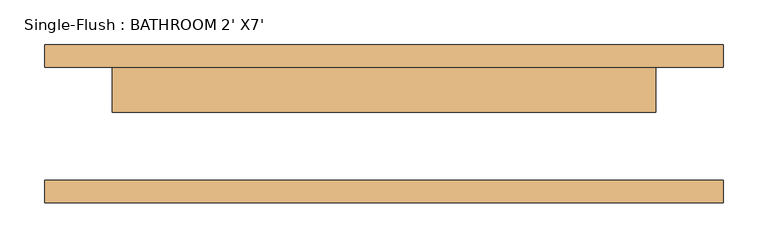
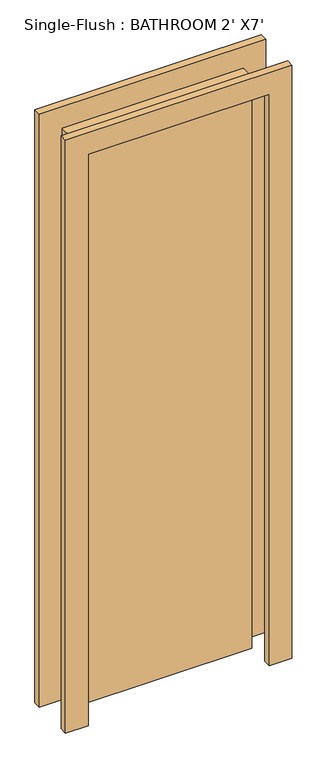
"""IFC4 building model written with IfcOpenShell, lengths in millimetres: door geometry, Single-Flush : BATHROOM 2' X7'."""

from ifc_helpers import new_model, si_unit, frame, origin, origin_with_axes, place, context, project, spatial, polyline, outline, extrude, source, transform, mapped, element, save


def single_flush_bathroom_2_x7_025d1c86(model_context):
    return source(origin(), model_context, "Body", "SweptSolid", [
        extrude(outline(polyline([(2108.2, -381.0), (0.0, -381.0), (0.0, -304.8), (2032.0, -304.8), (2032.0, 304.8), (0.0, 304.8), (0.0, 381.0), (2108.2, 381.0), (2108.2, -381.0)])), frame((0.0, 63.5, 0.0), z_axis=(0.0, 1.0, 0.0), x_axis=(0.0, 0.0, 1.0)), (0.0, 0.0, 1.0), 25.4),
        extrude(outline(polyline([(2108.2, 381.0), (2108.2, -381.0), (0.0, -381.0), (0.0, -304.8), (2032.0, -304.8), (2032.0, 304.8), (0.0, 304.8), (0.0, 381.0), (2108.2, 381.0)])), frame((0.0, -88.9, 0.0), z_axis=(0.0, 1.0, 0.0), x_axis=(0.0, 0.0, 1.0)), (0.0, 0.0, 1.0), 25.4),
        extrude(outline(polyline([(304.8, 12.7), (-304.8, 12.7), (-304.8, 63.5), (304.8, 63.5), (304.8, 12.7)])), origin_with_axes(), (0.0, 0.0, 1.0), 2032.0),
    ])


if __name__ == "__main__":
    model = new_model("IFC4")
    model_context = context("Model", 3, world=origin())
    ifc_project = project(units=[si_unit("LENGTHUNIT", "METRE", prefix="MILLI")], contexts=[model_context])
    site = spatial("IfcSite", under=ifc_project)
    building = spatial("IfcBuilding", under=site)
    placement = place(None, origin())
    single_flush_bathroom_2_x7_shape = single_flush_bathroom_2_x7_025d1c86(model_context)
    element("IfcDoor", 1, ObjectType="Single-Flush : BATHROOM 2' X7'", at=placement, inside=building, context=model_context, shape_type="MappedRepresentation", body=[
        mapped(single_flush_bathroom_2_x7_shape, transform((0.0, 0.0, 0.0), x_axis=(1.0, 0.0, 0.0), y_axis=(0.0, 1.0, 0.0), z_axis=(0.0, 0.0, 1.0))),
    ])
    save(model, "model.ifc")

# Revit data of these elements
# Type "Single-Flush : BATHROOM 2' X7'"
#   Type Mark = "12"
#   Construction Type Id = "MDOOR"
#   Assembly Code = "C1020"
#   Analytic Construction = "Metal"
#   Thickness = 0' - 2"
#   Heat Transfer Coefficient (U) = 0.651978 BTU/(h·ft²·°F)
#   Height = 6' - 8"
#   Trim Projection Ext = 0' - 1"
#   Trim Projection Int = 0' - 1"
#   Trim Width = 0' - 3"
#   Width = 2' - 0"
#   Define Thermal Properties by = 1
#   Door Material = Door - Panel
#   Frame Material = Door - Frame
#   Visual Light Transmittance = 0
#   Solar Heat Gain Coefficient = 0
#   Function = (empty or 0)
#   Wall Closure = (empty or 0)
# Element 1 (IfcDoor, "Single-Flush : BATHROOM 2' X7'")
#   Materials on its faces: "Door - Frame", "Door - Panel"
# Materials
#   "Door - Panel": class "Wood", colour RGB 210 159 95, transparency 0, Cost = 0
#   "Door - Frame": colour RGB 118 70 51, transparency 0, Cost = 0
